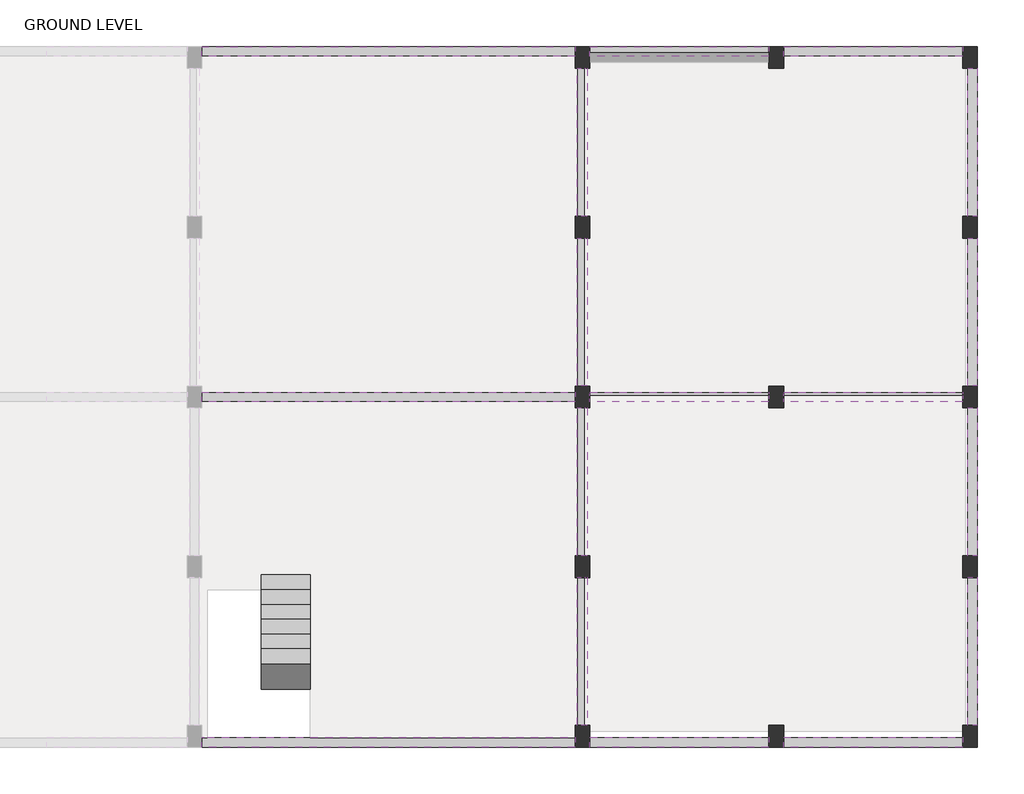
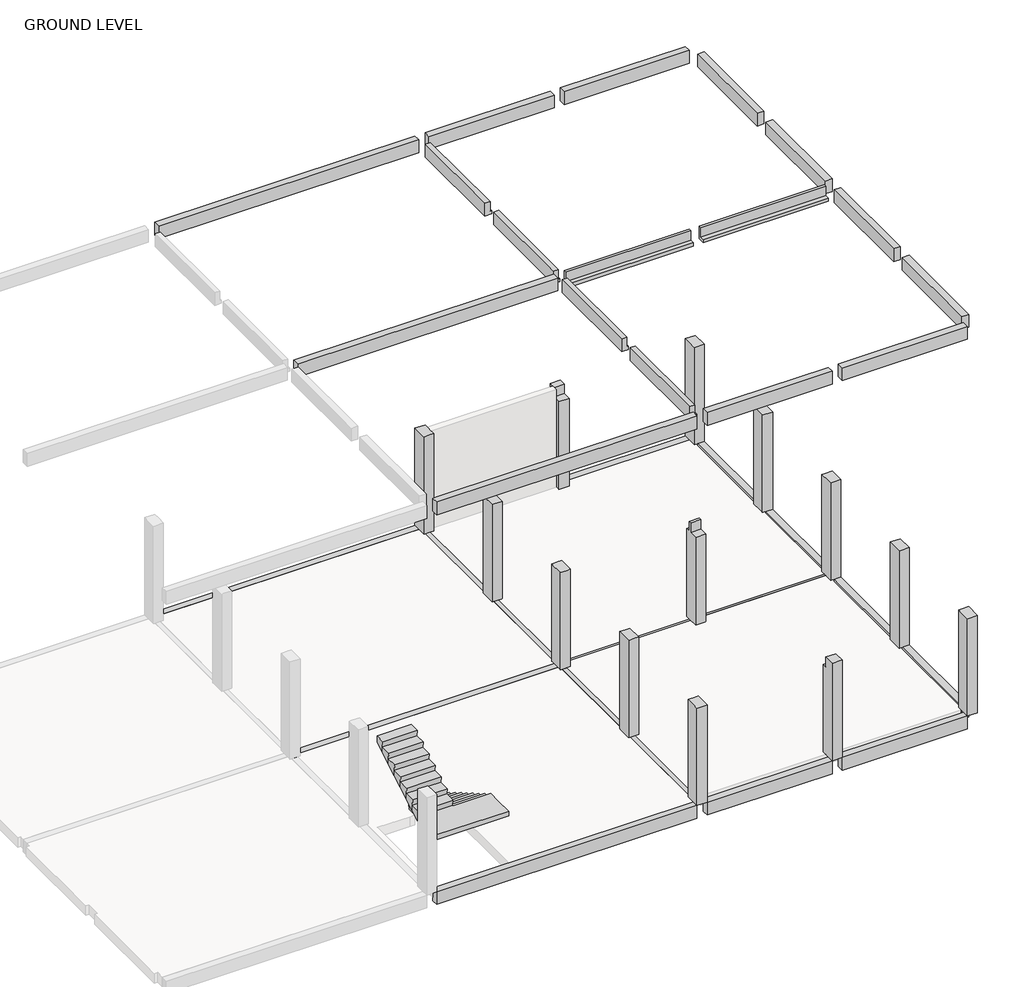
# One storey, part 2 of 2: 34 beams, 13 columns, 1 stair flight.
"""IFC4 building model written with IfcOpenShell, lengths in millimetres."""

from ifc_helpers import new_model, si_unit, frame, origin, place, context, project, spatial, polyline, outline, extrude, faceted_brep, element, save

model = new_model("IFC4")

# Units and contexts
model_context = context("Model", 3, world=origin())
ifc_project = project(units=[si_unit("LENGTHUNIT", "METRE", prefix="MILLI")], contexts=[model_context])

# Site, building, storey
site = spatial("IfcSite", under=ifc_project)
building = spatial("IfcBuilding", under=site)
storey = spatial("IfcBuildingStorey", under=building, Name="GROUND LEVEL", Elevation=0.0)

# Beams
placement = place(None, origin())
element("IfcBeam", 1, ObjectType="M_Concrete-Rectangular Beam : 200MMX400MM", at=placement, inside=storey, context=model_context, shape_type="Brep", body=[
    faceted_brep([(4019.3125983, 15797.7008557, 0.0), (4019.3125983, 15997.7008557, 0.0), (-3680.6874017, 15997.7008557, 0.0), (-3680.6874017, 15797.7008557, 0.0), (4019.3125983, 15797.7008557, -400.0), (4019.3125983, 15797.7008557, -300.0), (-3680.6874017, 15797.7008557, -300.0), (-3680.6874017, 15797.7008557, -400.0), (4019.3125983, 15997.7008557, -400.0), (-3680.6874017, 15997.7008557, -400.0)], [[[0, 1, 2, 3]], [[4, 5, 0, 3, 6, 7]], [[8, 4, 7, 9]], [[1, 8, 9, 2]], [[1, 0, 5, 4, 8]], [[2, 9, 7, 6, 3]]]),
])
element("IfcBeam", 2, ObjectType="M_Concrete-Rectangular Beam : 200MMX400MM", at=placement, inside=storey, context=model_context, shape_type="Brep", body=[
    faceted_brep([(8019.3125983, 15797.7008557, 0.0), (8019.3125983, 15997.7008557, 0.0), (4319.3125983, 15997.7008557, 0.0), (4319.3125983, 15797.7008557, 0.0), (8019.3125983, 15797.7008557, -400.0), (4319.3125983, 15797.7008557, -300.0), (4319.3125983, 15797.7008557, -400.0), (8019.3125983, 15997.7008557, -400.0), (4319.3125983, 15997.7008557, -400.0)], [[[0, 1, 2, 3]], [[4, 0, 3, 5, 6]], [[7, 4, 6, 8]], [[1, 7, 8, 2]], [[2, 8, 6, 5, 3]], [[1, 0, 4, 7]]]),
])
element("IfcBeam", 3, ObjectType="M_Concrete-Rectangular Beam : 200MMX400MM", at=placement, inside=storey, context=model_context, shape_type="Brep", body=[
    faceted_brep([(12019.3125983, 15797.7008557, 0.0), (12019.3125983, 15997.7008557, 0.0), (8319.3125983, 15997.7008557, 0.0), (8319.3125983, 15797.7008557, 0.0), (12019.3125983, 15797.7008557, -400.0), (12019.3125983, 15797.7008557, -300.0), (8319.3125983, 15797.7008557, -400.0), (12019.3125983, 15997.7008557, -400.0), (8319.3125983, 15997.7008557, -400.0)], [[[0, 1, 2, 3]], [[4, 5, 0, 3, 6]], [[7, 4, 6, 8]], [[1, 7, 8, 2]], [[2, 8, 6, 3]], [[1, 0, 5, 4, 7]]]),
])
element("IfcBeam", 4, ObjectType="M_Concrete-Rectangular Beam : 200MMX400MM", at=placement, inside=storey, context=model_context, shape_type="SweptSolid", body=[
    extrude(outline(polyline([(12319.3125983, 12497.7008557), (12119.3125983, 12497.7008557), (12119.3125983, 15547.7008557), (12319.3125983, 15547.7008557), (12319.3125983, 12497.7008557)])), frame((0.0, 0.0, -400.0), z_axis=(0.0, 0.0, 1.0), x_axis=(1.0, 0.0, 0.0)), (0.0, 0.0, 1.0), 400.0),
])
element("IfcBeam", 5, ObjectType="M_Concrete-Rectangular Beam : 200MMX400MM", at=placement, inside=storey, context=model_context, shape_type="SweptSolid", body=[
    extrude(outline(polyline([(12319.3125983, 1997.7008557), (12119.3125983, 1997.7008557), (12119.3125983, 5047.7008557), (12319.3125983, 5047.7008557), (12319.3125983, 1997.7008557)])), frame((0.0, 0.0, -400.0), z_axis=(0.0, 0.0, 1.0), x_axis=(1.0, 0.0, 0.0)), (0.0, 0.0, 1.0), 400.0),
])
element("IfcBeam", 6, ObjectType="M_Concrete-Rectangular Beam : 200MMX400MM", at=placement, inside=storey, context=model_context, shape_type="SweptSolid", body=[
    extrude(outline(polyline([(8319.3125983, 1547.7008557), (8319.3125983, 1747.7008557), (12019.3125983, 1747.7008557), (12019.3125983, 1547.7008557), (8319.3125983, 1547.7008557)])), frame((0.0, 0.0, -400.0), z_axis=(0.0, 0.0, 1.0), x_axis=(1.0, 0.0, 0.0)), (0.0, 0.0, 1.0), 400.0),
])
element("IfcBeam", 7, ObjectType="M_Concrete-Rectangular Beam : 200MMX400MM", at=placement, inside=storey, context=model_context, shape_type="SweptSolid", body=[
    extrude(outline(polyline([(8019.3125983, 1747.7008557), (8019.3125983, 1547.7008557), (4319.3125983, 1547.7008557), (4319.3125983, 1747.7008557), (8019.3125983, 1747.7008557)])), frame((0.0, 0.0, -400.0), z_axis=(0.0, 0.0, 1.0), x_axis=(1.0, 0.0, 0.0)), (0.0, 0.0, 1.0), 400.0),
])
element("IfcBeam", 8, ObjectType="M_Concrete-Rectangular Beam : 200MMX400MM", at=placement, inside=storey, context=model_context, shape_type="Brep", body=[
    faceted_brep([(-3680.6874017, 1747.7008557, 0.0), (-3680.6874017, 1547.7008557, 0.0), (4019.3125983, 1547.7008557, 0.0), (4019.3125983, 1747.7008557, 0.0), (-1437.0874017, 1747.7008557, 0.0), (-3570.6874017, 1747.7008557, 0.0), (-3680.6874017, 1747.7008557, -400.0), (-3680.6874017, 1747.7008557, -300.0), (4019.3125983, 1747.7008557, -300.0), (4019.3125983, 1747.7008557, -400.0), (-3680.6874017, 1547.7008557, -400.0), (4019.3125983, 1547.7008557, -400.0)], [[[0, 1, 2, 3, 4, 5]], [[6, 7, 0, 5, 4, 3, 8, 9]], [[10, 6, 9, 11]], [[1, 10, 11, 2]], [[1, 0, 7, 6, 10]], [[2, 11, 9, 8, 3]]]),
])
element("IfcBeam", 9, ObjectType="M_Concrete-Rectangular Beam : 200MMX400MM", at=placement, inside=storey, context=model_context, shape_type="Brep", body=[
    faceted_brep([(4019.3125983, 8872.7008557, 0.0), (-3680.6874017, 8872.7008557, 0.0), (-3680.6874017, 8672.7008557, 0.0), (4019.3125983, 8672.7008557, 0.0), (-3680.6874017, 8672.7008557, -300.0), (-3680.6874017, 8672.7008557, -400.0), (4019.3125983, 8672.7008557, -400.0), (4019.3125983, 8672.7008557, -300.0), (-3680.6874017, 8872.7008557, -400.0), (4019.3125983, 8872.7008557, -400.0), (4019.3125983, 8872.7008557, -300.0), (-3680.6874017, 8872.7008557, -300.0)], [[[0, 1, 2, 3]], [[3, 2, 4, 5, 6, 7]], [[6, 5, 8, 9]], [[1, 0, 10, 9, 8, 11]], [[8, 5, 4, 2, 1, 11]], [[0, 3, 7, 6, 9, 10]]]),
])
element("IfcBeam", 10, ObjectType="M_Concrete-Rectangular Beam : 200MMX400MM", at=placement, inside=storey, context=model_context, shape_type="Brep", body=[
    faceted_brep([(8019.3125983, 8872.7008557, 0.0), (4319.3125983, 8872.7008557, 0.0), (4319.3125983, 8797.7008557, 0.0), (8019.3125983, 8797.7008557, 0.0), (4319.3125983, 8672.7008557, -400.0), (8019.3125983, 8672.7008557, -400.0), (8019.3125983, 8672.7008557, -300.0), (4319.3125983, 8672.7008557, -300.0), (4319.3125983, 8872.7008557, -400.0), (8019.3125983, 8872.7008557, -400.0), (8019.3125983, 8872.7008557, -300.0), (4319.3125983, 8872.7008557, -300.0), (4319.3125983, 8797.7008557, -300.0), (8019.3125983, 8797.7008557, -300.0)], [[[0, 1, 2, 3]], [[4, 5, 6, 7]], [[5, 4, 8, 9]], [[1, 0, 10, 9, 8, 11]], [[8, 4, 7, 12, 2, 1, 11]], [[5, 9, 10, 0, 3, 13, 6]], [[13, 12, 7, 6]], [[12, 13, 3, 2]]]),
])
element("IfcBeam", 11, ObjectType="M_Concrete-Rectangular Beam : 200MMX400MM", at=placement, inside=storey, context=model_context, shape_type="Brep", body=[
    faceted_brep([(12019.3125983, 8872.7008557, 0.0), (8319.3125983, 8872.7008557, 0.0), (8319.3125983, 8797.7008557, 0.0), (12019.3125983, 8797.7008557, 0.0), (8319.3125983, 8672.7008557, -400.0), (12019.3125983, 8672.7008557, -400.0), (12019.3125983, 8672.7008557, -300.0), (8319.3125983, 8672.7008557, -300.0), (8319.3125983, 8872.7008557, -400.0), (12019.3125983, 8872.7008557, -400.0), (12019.3125983, 8872.7008557, -300.0), (8319.3125983, 8872.7008557, -300.0), (12019.3125983, 8797.7008557, -300.0), (8319.3125983, 8797.7008557, -300.0)], [[[0, 1, 2, 3]], [[4, 5, 6, 7]], [[5, 4, 8, 9]], [[1, 0, 10, 9, 8, 11]], [[5, 9, 10, 0, 3, 12, 6]], [[8, 4, 7, 13, 2, 1, 11]], [[12, 13, 7, 6]], [[13, 12, 3, 2]]]),
])
element("IfcBeam", 12, ObjectType="M_Concrete-Rectangular Beam : 200MMX400MM", at=placement, inside=storey, context=model_context, shape_type="SweptSolid", body=[
    extrude(outline(polyline([(12319.3125983, 5497.7008557), (12119.3125983, 5497.7008557), (12119.3125983, 8547.7008557), (12319.3125983, 8547.7008557), (12319.3125983, 5497.7008557)])), frame((0.0, 0.0, -400.0), z_axis=(0.0, 0.0, 1.0), x_axis=(1.0, 0.0, 0.0)), (0.0, 0.0, 1.0), 400.0),
])
element("IfcBeam", 13, ObjectType="M_Concrete-Rectangular Beam : 200MMX400MM", at=placement, inside=storey, context=model_context, shape_type="SweptSolid", body=[
    extrude(outline(polyline([(12119.3125983, 12047.7008557), (12319.3125983, 12047.7008557), (12319.3125983, 8997.7008557), (12119.3125983, 8997.7008557), (12119.3125983, 12047.7008557)])), frame((0.0, 0.0, -400.0), z_axis=(0.0, 0.0, 1.0), x_axis=(1.0, 0.0, 0.0)), (0.0, 0.0, 1.0), 400.0),
])
element("IfcBeam", 14, ObjectType="M_Concrete-Rectangular Beam : 200MMX400MM", at=placement, inside=storey, context=model_context, shape_type="Brep", body=[
    faceted_brep([(4069.3125983, 5047.7008557, 0.0), (4069.3125983, 1997.7008557, 0.0), (4219.3125983, 1997.7008557, 0.0), (4219.3125983, 5047.7008557, 0.0), (4269.3125983, 1997.7008557, -400.0), (4269.3125983, 5047.7008557, -400.0), (4269.3125983, 5047.7008557, -300.0), (4269.3125983, 1997.7008557, -300.0), (4069.3125983, 1997.7008557, -400.0), (4069.3125983, 5047.7008557, -400.0), (4069.3125983, 5047.7008557, -300.0), (4069.3125983, 1997.7008557, -300.0), (4219.3125983, 1997.7008557, -300.0), (4219.3125983, 5047.7008557, -300.0)], [[[0, 1, 2, 3]], [[4, 5, 6, 7]], [[5, 4, 8, 9]], [[1, 0, 10, 9, 8, 11]], [[8, 4, 7, 12, 2, 1, 11]], [[5, 9, 10, 0, 3, 13, 6]], [[13, 12, 7, 6]], [[12, 13, 3, 2]]]),
])
element("IfcBeam", 15, ObjectType="M_Concrete-Rectangular Beam : 200MMX400MM", at=placement, inside=storey, context=model_context, shape_type="Brep", body=[
    faceted_brep([(4069.3125983, 8547.7008557, 0.0), (4069.3125983, 5497.7008557, 0.0), (4219.3125983, 5497.7008557, 0.0), (4219.3125983, 8547.7008557, 0.0), (4269.3125983, 5497.7008557, -400.0), (4269.3125983, 8547.7008557, -400.0), (4269.3125983, 8547.7008557, -300.0), (4269.3125983, 5497.7008557, -300.0), (4069.3125983, 5497.7008557, -400.0), (4069.3125983, 8547.7008557, -400.0), (4069.3125983, 8547.7008557, -300.0), (4069.3125983, 5497.7008557, -300.0), (4219.3125983, 8547.7008557, -300.0), (4219.3125983, 5497.7008557, -300.0)], [[[0, 1, 2, 3]], [[4, 5, 6, 7]], [[5, 4, 8, 9]], [[1, 0, 10, 9, 8, 11]], [[5, 9, 10, 0, 3, 12, 6]], [[8, 4, 7, 13, 2, 1, 11]], [[12, 13, 7, 6]], [[13, 12, 3, 2]]]),
])
element("IfcBeam", 16, ObjectType="M_Concrete-Rectangular Beam : 200MMX400MM", at=placement, inside=storey, context=model_context, shape_type="Brep", body=[
    faceted_brep([(4069.3125983, 12047.7008557, 0.0), (4069.3125983, 8997.7008557, 0.0), (4219.3125983, 8997.7008557, 0.0), (4219.3125983, 12047.7008557, 0.0), (4269.3125983, 8997.7008557, -400.0), (4269.3125983, 12047.7008557, -400.0), (4269.3125983, 12047.7008557, -300.0), (4269.3125983, 8997.7008557, -300.0), (4069.3125983, 8997.7008557, -400.0), (4069.3125983, 12047.7008557, -400.0), (4069.3125983, 12047.7008557, -300.0), (4069.3125983, 8997.7008557, -300.0), (4219.3125983, 8997.7008557, -300.0), (4219.3125983, 12047.7008557, -300.0)], [[[0, 1, 2, 3]], [[4, 5, 6, 7]], [[5, 4, 8, 9]], [[1, 0, 10, 9, 8, 11]], [[8, 4, 7, 12, 2, 1, 11]], [[5, 9, 10, 0, 3, 13, 6]], [[13, 12, 7, 6]], [[12, 13, 3, 2]]]),
])
element("IfcBeam", 17, ObjectType="M_Concrete-Rectangular Beam : 200MMX400MM", at=placement, inside=storey, context=model_context, shape_type="Brep", body=[
    faceted_brep([(4069.3125983, 15547.7008557, 0.0), (4069.3125983, 12497.7008557, 0.0), (4219.3125983, 12497.7008557, 0.0), (4219.3125983, 15547.7008557, 0.0), (4269.3125983, 12497.7008557, -400.0), (4269.3125983, 15547.7008557, -400.0), (4269.3125983, 15547.7008557, -300.0), (4269.3125983, 12497.7008557, -300.0), (4069.3125983, 12497.7008557, -400.0), (4069.3125983, 15547.7008557, -400.0), (4069.3125983, 15547.7008557, -300.0), (4069.3125983, 12497.7008557, -300.0), (4219.3125983, 15547.7008557, -300.0), (4219.3125983, 12497.7008557, -300.0)], [[[0, 1, 2, 3]], [[4, 5, 6, 7]], [[5, 4, 8, 9]], [[1, 0, 10, 9, 8, 11]], [[5, 9, 10, 0, 3, 12, 6]], [[8, 4, 7, 13, 2, 1, 11]], [[12, 13, 7, 6]], [[13, 12, 3, 2]]]),
])
element("IfcBeam", 18, ObjectType="M_Concrete-Rectangular Beam : 200MMX400MM", at=placement, inside=storey, context=model_context, shape_type="Brep", body=[
    faceted_brep([(4019.3125983, 15797.7008557, 12192.0), (4019.3125983, 15997.7008557, 12192.0), (-3680.6874017, 15997.7008557, 12192.0), (-3680.6874017, 15797.7008557, 12192.0), (4019.3125983, 15797.7008557, 11792.0), (4019.3125983, 15797.7008557, 11892.0), (-3680.6874017, 15797.7008557, 11892.0), (-3680.6874017, 15797.7008557, 11792.0), (4019.3125983, 15997.7008557, 11792.0), (-3680.6874017, 15997.7008557, 11792.0)], [[[0, 1, 2, 3]], [[4, 5, 0, 3, 6, 7]], [[8, 4, 7, 9]], [[1, 8, 9, 2]], [[1, 0, 5, 4, 8]], [[2, 9, 7, 6, 3]]]),
])
element("IfcBeam", 19, ObjectType="M_Concrete-Rectangular Beam : 200MMX400MM", at=placement, inside=storey, context=model_context, shape_type="Brep", body=[
    faceted_brep([(8019.3125983, 15797.7008557, 12192.0), (8019.3125983, 15997.7008557, 12192.0), (4319.3125983, 15997.7008557, 12192.0), (4319.3125983, 15797.7008557, 12192.0), (8019.3125983, 15797.7008557, 11792.0), (4319.3125983, 15797.7008557, 11892.0), (4319.3125983, 15797.7008557, 11792.0), (8019.3125983, 15997.7008557, 11792.0), (4319.3125983, 15997.7008557, 11792.0)], [[[0, 1, 2, 3]], [[4, 0, 3, 5, 6]], [[7, 4, 6, 8]], [[1, 7, 8, 2]], [[2, 8, 6, 5, 3]], [[1, 0, 4, 7]]]),
])
element("IfcBeam", 20, ObjectType="M_Concrete-Rectangular Beam : 200MMX400MM", at=placement, inside=storey, context=model_context, shape_type="Brep", body=[
    faceted_brep([(12019.3125983, 15797.7008557, 12192.0), (12019.3125983, 15997.7008557, 12192.0), (8319.3125983, 15997.7008557, 12192.0), (8319.3125983, 15797.7008557, 12192.0), (12019.3125983, 15797.7008557, 11792.0), (12019.3125983, 15797.7008557, 11892.0), (8319.3125983, 15797.7008557, 11792.0), (12019.3125983, 15997.7008557, 11792.0), (8319.3125983, 15997.7008557, 11792.0)], [[[0, 1, 2, 3]], [[4, 5, 0, 3, 6]], [[7, 4, 6, 8]], [[1, 7, 8, 2]], [[2, 8, 6, 3]], [[1, 0, 5, 4, 7]]]),
])
element("IfcBeam", 21, ObjectType="M_Concrete-Rectangular Beam : 200MMX400MM", at=placement, inside=storey, context=model_context, shape_type="SweptSolid", body=[
    extrude(outline(polyline([(12319.3125983, 12497.7008557), (12119.3125983, 12497.7008557), (12119.3125983, 15547.7008557), (12319.3125983, 15547.7008557), (12319.3125983, 12497.7008557)])), frame((0.0, 0.0, 11792.0), z_axis=(0.0, 0.0, 1.0), x_axis=(1.0, 0.0, 0.0)), (0.0, 0.0, 1.0), 400.0),
])
element("IfcBeam", 22, ObjectType="M_Concrete-Rectangular Beam : 200MMX400MM", at=placement, inside=storey, context=model_context, shape_type="SweptSolid", body=[
    extrude(outline(polyline([(12319.3125983, 1997.7008557), (12119.3125983, 1997.7008557), (12119.3125983, 5047.7008557), (12319.3125983, 5047.7008557), (12319.3125983, 1997.7008557)])), frame((0.0, 0.0, 11792.0), z_axis=(0.0, 0.0, 1.0), x_axis=(1.0, 0.0, 0.0)), (0.0, 0.0, 1.0), 400.0),
])
element("IfcBeam", 23, ObjectType="M_Concrete-Rectangular Beam : 200MMX400MM", at=placement, inside=storey, context=model_context, shape_type="SweptSolid", body=[
    extrude(outline(polyline([(8319.3125983, 1547.7008557), (8319.3125983, 1747.7008557), (12019.3125983, 1747.7008557), (12019.3125983, 1547.7008557), (8319.3125983, 1547.7008557)])), frame((0.0, 0.0, 11792.0), z_axis=(0.0, 0.0, 1.0), x_axis=(1.0, 0.0, 0.0)), (0.0, 0.0, 1.0), 400.0),
])
element("IfcBeam", 24, ObjectType="M_Concrete-Rectangular Beam : 200MMX400MM", at=placement, inside=storey, context=model_context, shape_type="SweptSolid", body=[
    extrude(outline(polyline([(8019.3125983, 1747.7008557), (8019.3125983, 1547.7008557), (4319.3125983, 1547.7008557), (4319.3125983, 1747.7008557), (8019.3125983, 1747.7008557)])), frame((0.0, 0.0, 11792.0), z_axis=(0.0, 0.0, 1.0), x_axis=(1.0, 0.0, 0.0)), (0.0, 0.0, 1.0), 400.0),
])
element("IfcBeam", 25, ObjectType="M_Concrete-Rectangular Beam : 200MMX400MM", at=placement, inside=storey, context=model_context, shape_type="Brep", body=[
    faceted_brep([(-3680.6874017, 1747.7008557, 12192.0), (-3680.6874017, 1547.7008557, 12192.0), (4019.3125983, 1547.7008557, 12192.0), (4019.3125983, 1747.7008557, 12192.0), (-1437.0874017, 1747.7008557, 12192.0), (-3570.6874017, 1747.7008557, 12192.0), (-3680.6874017, 1747.7008557, 11792.0), (-3680.6874017, 1747.7008557, 11892.0), (4019.3125983, 1747.7008557, 11892.0), (4019.3125983, 1747.7008557, 11792.0), (-3680.6874017, 1547.7008557, 11792.0), (4019.3125983, 1547.7008557, 11792.0)], [[[0, 1, 2, 3, 4, 5]], [[6, 7, 0, 5, 4, 3, 8, 9]], [[10, 6, 9, 11]], [[1, 10, 11, 2]], [[1, 0, 7, 6, 10]], [[2, 11, 9, 8, 3]]]),
])
element("IfcBeam", 26, ObjectType="M_Concrete-Rectangular Beam : 200MMX400MM", at=placement, inside=storey, context=model_context, shape_type="Brep", body=[
    faceted_brep([(4019.3125983, 8872.7008557, 12192.0), (-3680.6874017, 8872.7008557, 12192.0), (-3680.6874017, 8672.7008557, 12192.0), (4019.3125983, 8672.7008557, 12192.0), (-3680.6874017, 8672.7008557, 11892.0), (-3680.6874017, 8672.7008557, 11792.0), (4019.3125983, 8672.7008557, 11792.0), (4019.3125983, 8672.7008557, 11892.0), (-3680.6874017, 8872.7008557, 11792.0), (4019.3125983, 8872.7008557, 11792.0), (4019.3125983, 8872.7008557, 11892.0), (-3680.6874017, 8872.7008557, 11892.0)], [[[0, 1, 2, 3]], [[3, 2, 4, 5, 6, 7]], [[6, 5, 8, 9]], [[1, 0, 10, 9, 8, 11]], [[8, 5, 4, 2, 1, 11]], [[0, 3, 7, 6, 9, 10]]]),
])
element("IfcBeam", 27, ObjectType="M_Concrete-Rectangular Beam : 200MMX400MM", at=placement, inside=storey, context=model_context, shape_type="Brep", body=[
    faceted_brep([(8019.3125983, 8872.7008557, 12192.0), (4319.3125983, 8872.7008557, 12192.0), (4319.3125983, 8797.7008557, 12192.0), (8019.3125983, 8797.7008557, 12192.0), (4319.3125983, 8672.7008557, 11792.0), (8019.3125983, 8672.7008557, 11792.0), (8019.3125983, 8672.7008557, 11892.0), (4319.3125983, 8672.7008557, 11892.0), (4319.3125983, 8872.7008557, 11792.0), (8019.3125983, 8872.7008557, 11792.0), (8019.3125983, 8872.7008557, 11892.0), (4319.3125983, 8872.7008557, 11892.0), (4319.3125983, 8797.7008557, 11892.0), (8019.3125983, 8797.7008557, 11892.0)], [[[0, 1, 2, 3]], [[4, 5, 6, 7]], [[5, 4, 8, 9]], [[1, 0, 10, 9, 8, 11]], [[8, 4, 7, 12, 2, 1, 11]], [[5, 9, 10, 0, 3, 13, 6]], [[13, 12, 7, 6]], [[12, 13, 3, 2]]]),
])
element("IfcBeam", 28, ObjectType="M_Concrete-Rectangular Beam : 200MMX400MM", at=placement, inside=storey, context=model_context, shape_type="Brep", body=[
    faceted_brep([(12019.3125983, 8872.7008557, 12192.0), (8319.3125983, 8872.7008557, 12192.0), (8319.3125983, 8797.7008557, 12192.0), (12019.3125983, 8797.7008557, 12192.0), (8319.3125983, 8672.7008557, 11792.0), (12019.3125983, 8672.7008557, 11792.0), (12019.3125983, 8672.7008557, 11892.0), (8319.3125983, 8672.7008557, 11892.0), (8319.3125983, 8872.7008557, 11792.0), (12019.3125983, 8872.7008557, 11792.0), (12019.3125983, 8872.7008557, 11892.0), (8319.3125983, 8872.7008557, 11892.0), (12019.3125983, 8797.7008557, 11892.0), (8319.3125983, 8797.7008557, 11892.0)], [[[0, 1, 2, 3]], [[4, 5, 6, 7]], [[5, 4, 8, 9]], [[1, 0, 10, 9, 8, 11]], [[5, 9, 10, 0, 3, 12, 6]], [[8, 4, 7, 13, 2, 1, 11]], [[12, 13, 7, 6]], [[13, 12, 3, 2]]]),
])
element("IfcBeam", 29, ObjectType="M_Concrete-Rectangular Beam : 200MMX400MM", at=placement, inside=storey, context=model_context, shape_type="SweptSolid", body=[
    extrude(outline(polyline([(12319.3125983, 5497.7008557), (12119.3125983, 5497.7008557), (12119.3125983, 8547.7008557), (12319.3125983, 8547.7008557), (12319.3125983, 5497.7008557)])), frame((0.0, 0.0, 11792.0), z_axis=(0.0, 0.0, 1.0), x_axis=(1.0, 0.0, 0.0)), (0.0, 0.0, 1.0), 400.0),
])
element("IfcBeam", 30, ObjectType="M_Concrete-Rectangular Beam : 200MMX400MM", at=placement, inside=storey, context=model_context, shape_type="SweptSolid", body=[
    extrude(outline(polyline([(12119.3125983, 12047.7008557), (12319.3125983, 12047.7008557), (12319.3125983, 8997.7008557), (12119.3125983, 8997.7008557), (12119.3125983, 12047.7008557)])), frame((0.0, 0.0, 11792.0), z_axis=(0.0, 0.0, 1.0), x_axis=(1.0, 0.0, 0.0)), (0.0, 0.0, 1.0), 400.0),
])
element("IfcBeam", 31, ObjectType="M_Concrete-Rectangular Beam : 200MMX400MM", at=placement, inside=storey, context=model_context, shape_type="Brep", body=[
    faceted_brep([(4069.3125983, 5047.7008557, 12192.0), (4069.3125983, 1997.7008557, 12192.0), (4219.3125983, 1997.7008557, 12192.0), (4219.3125983, 5047.7008557, 12192.0), (4269.3125983, 1997.7008557, 11792.0), (4269.3125983, 5047.7008557, 11792.0), (4269.3125983, 5047.7008557, 11892.0), (4269.3125983, 1997.7008557, 11892.0), (4069.3125983, 1997.7008557, 11792.0), (4069.3125983, 5047.7008557, 11792.0), (4069.3125983, 5047.7008557, 11892.0), (4069.3125983, 1997.7008557, 11892.0), (4219.3125983, 1997.7008557, 11892.0), (4219.3125983, 5047.7008557, 11892.0)], [[[0, 1, 2, 3]], [[4, 5, 6, 7]], [[5, 4, 8, 9]], [[1, 0, 10, 9, 8, 11]], [[8, 4, 7, 12, 2, 1, 11]], [[5, 9, 10, 0, 3, 13, 6]], [[13, 12, 7, 6]], [[12, 13, 3, 2]]]),
])
element("IfcBeam", 32, ObjectType="M_Concrete-Rectangular Beam : 200MMX400MM", at=placement, inside=storey, context=model_context, shape_type="Brep", body=[
    faceted_brep([(4069.3125983, 8547.7008557, 12192.0), (4069.3125983, 5497.7008557, 12192.0), (4219.3125983, 5497.7008557, 12192.0), (4219.3125983, 8547.7008557, 12192.0), (4269.3125983, 5497.7008557, 11792.0), (4269.3125983, 8547.7008557, 11792.0), (4269.3125983, 8547.7008557, 11892.0), (4269.3125983, 5497.7008557, 11892.0), (4069.3125983, 5497.7008557, 11792.0), (4069.3125983, 8547.7008557, 11792.0), (4069.3125983, 8547.7008557, 11892.0), (4069.3125983, 5497.7008557, 11892.0), (4219.3125983, 8547.7008557, 11892.0), (4219.3125983, 5497.7008557, 11892.0)], [[[0, 1, 2, 3]], [[4, 5, 6, 7]], [[5, 4, 8, 9]], [[1, 0, 10, 9, 8, 11]], [[5, 9, 10, 0, 3, 12, 6]], [[8, 4, 7, 13, 2, 1, 11]], [[12, 13, 7, 6]], [[13, 12, 3, 2]]]),
])
element("IfcBeam", 33, ObjectType="M_Concrete-Rectangular Beam : 200MMX400MM", at=placement, inside=storey, context=model_context, shape_type="Brep", body=[
    faceted_brep([(4069.3125983, 12047.7008557, 12192.0), (4069.3125983, 8997.7008557, 12192.0), (4219.3125983, 8997.7008557, 12192.0), (4219.3125983, 12047.7008557, 12192.0), (4269.3125983, 8997.7008557, 11792.0), (4269.3125983, 12047.7008557, 11792.0), (4269.3125983, 12047.7008557, 11892.0), (4269.3125983, 8997.7008557, 11892.0), (4069.3125983, 8997.7008557, 11792.0), (4069.3125983, 12047.7008557, 11792.0), (4069.3125983, 12047.7008557, 11892.0), (4069.3125983, 8997.7008557, 11892.0), (4219.3125983, 8997.7008557, 11892.0), (4219.3125983, 12047.7008557, 11892.0)], [[[0, 1, 2, 3]], [[4, 5, 6, 7]], [[5, 4, 8, 9]], [[1, 0, 10, 9, 8, 11]], [[8, 4, 7, 12, 2, 1, 11]], [[5, 9, 10, 0, 3, 13, 6]], [[13, 12, 7, 6]], [[12, 13, 3, 2]]]),
])
element("IfcBeam", 34, ObjectType="M_Concrete-Rectangular Beam : 200MMX400MM", at=placement, inside=storey, context=model_context, shape_type="Brep", body=[
    faceted_brep([(4069.3125983, 15547.7008557, 12192.0), (4069.3125983, 12497.7008557, 12192.0), (4219.3125983, 12497.7008557, 12192.0), (4219.3125983, 15547.7008557, 12192.0), (4269.3125983, 12497.7008557, 11792.0), (4269.3125983, 15547.7008557, 11792.0), (4269.3125983, 15547.7008557, 11892.0), (4269.3125983, 12497.7008557, 11892.0), (4069.3125983, 12497.7008557, 11792.0), (4069.3125983, 15547.7008557, 11792.0), (4069.3125983, 15547.7008557, 11892.0), (4069.3125983, 12497.7008557, 11892.0), (4219.3125983, 15547.7008557, 11892.0), (4219.3125983, 12497.7008557, 11892.0)], [[[0, 1, 2, 3]], [[4, 5, 6, 7]], [[5, 4, 8, 9]], [[1, 0, 10, 9, 8, 11]], [[5, 9, 10, 0, 3, 12, 6]], [[8, 4, 7, 13, 2, 1, 11]], [[12, 13, 7, 6]], [[13, 12, 3, 2]]]),
])

# Columns
element("IfcColumn", 35, ObjectType="M_Concrete-Rectangular-Column : 300 x 450mm", at=placement, inside=storey, context=model_context, shape_type="Brep", body=[
    faceted_brep([(4319.3125983, 15997.7008557, 0.0), (4319.3125983, 15547.7008557, 0.0), (4019.3125983, 15547.7008557, 0.0), (4019.3125983, 15997.7008557, 0.0), (4319.3125983, 15997.7008557, 3048.0), (4319.3125983, 15797.7008557, 3048.0), (4319.3125983, 15547.7008557, 3048.0), (4319.3125983, 15547.7008557, 2748.0), (4219.3125983, 15547.7008557, 3048.0), (4069.3125983, 15547.7008557, 3048.0), (4019.3125983, 15547.7008557, 3048.0), (4019.3125983, 15547.7008557, 2748.0), (4019.3125983, 15797.7008557, 3048.0), (4019.3125983, 15997.7008557, 3048.0)], [[[0, 1, 2, 3]], [[1, 0, 4, 5, 6, 7]], [[2, 1, 7, 6, 8, 9, 10, 11]], [[3, 2, 11, 10, 12, 13]], [[0, 3, 13, 4]], [[4, 13, 12, 10, 9, 8, 6, 5]]]),
])
element("IfcColumn", 36, ObjectType="M_Concrete-Rectangular-Column : 300 x 450mm", at=placement, inside=storey, context=model_context, shape_type="Brep", body=[
    faceted_brep([(4319.3125983, 8997.7008557, 0.0), (4319.3125983, 8547.7008557, 0.0), (4019.3125983, 8547.7008557, 0.0), (4019.3125983, 8997.7008557, 0.0), (4319.3125983, 8997.7008557, 2748.0), (4319.3125983, 8997.7008557, 3048.0), (4319.3125983, 8872.7008557, 3048.0), (4319.3125983, 8797.7008557, 3048.0), (4319.3125983, 8547.7008557, 3048.0), (4319.3125983, 8547.7008557, 2748.0), (4219.3125983, 8547.7008557, 3048.0), (4069.3125983, 8547.7008557, 3048.0), (4019.3125983, 8547.7008557, 3048.0), (4019.3125983, 8547.7008557, 2748.0), (4019.3125983, 8672.7008557, 3048.0), (4019.3125983, 8872.7008557, 3048.0), (4019.3125983, 8997.7008557, 3048.0), (4019.3125983, 8997.7008557, 2748.0), (4069.3125983, 8997.7008557, 3048.0), (4219.3125983, 8997.7008557, 3048.0)], [[[0, 1, 2, 3]], [[1, 0, 4, 5, 6, 7, 8, 9]], [[2, 1, 9, 8, 10, 11, 12, 13]], [[3, 2, 13, 12, 14, 15, 16, 17]], [[0, 3, 17, 16, 18, 19, 5, 4]], [[18, 16, 15, 14, 12, 11, 10, 8, 7, 6, 5, 19]]]),
])
element("IfcColumn", 37, ObjectType="M_Concrete-Rectangular-Column : 300 x 450mm", at=placement, inside=storey, context=model_context, shape_type="Brep", body=[
    faceted_brep([(4319.3125983, 1997.7008557, 0.0), (4319.3125983, 1547.7008557, 0.0), (4019.3125983, 1547.7008557, 0.0), (4019.3125983, 1997.7008557, 0.0), (4319.3125983, 1997.7008557, 2748.0), (4319.3125983, 1997.7008557, 3048.0), (4319.3125983, 1872.7008557, 3048.0), (4319.3125983, 1547.7008557, 3048.0), (4019.3125983, 1547.7008557, 3048.0), (4019.3125983, 1747.7008557, 3048.0), (4019.3125983, 1997.7008557, 3048.0), (4019.3125983, 1997.7008557, 2748.0), (4069.3125983, 1997.7008557, 3048.0), (4219.3125983, 1997.7008557, 3048.0)], [[[0, 1, 2, 3]], [[1, 0, 4, 5, 6, 7]], [[2, 1, 7, 8]], [[3, 2, 8, 9, 10, 11]], [[0, 3, 11, 10, 12, 13, 5, 4]], [[8, 7, 6, 5, 13, 12, 10, 9]]]),
])
element("IfcColumn", 38, ObjectType="M_Concrete-Rectangular-Column : 300 x 450mm", at=placement, inside=storey, context=model_context, shape_type="SweptSolid", body=[
    extrude(outline(polyline([(15997.7008557, 0.0), (15547.7008557, 0.0), (15547.7008557, 2748.0), (15797.7008557, 2748.0), (15797.7008557, 3048.0), (15997.7008557, 3048.0), (15997.7008557, 0.0)])), frame((8019.3125983, 0.0, 0.0), z_axis=(1.0, 0.0, 0.0), x_axis=(0.0, 1.0, 0.0)), (0.0, 0.0, 1.0), 300.0),
])
element("IfcColumn", 39, ObjectType="M_Concrete-Rectangular-Column : 300 x 450mm", at=placement, inside=storey, context=model_context, shape_type="SweptSolid", body=[
    extrude(outline(polyline([(1997.7008557, 0.0), (1547.7008557, 0.0), (1547.7008557, 3048.0), (1872.7008557, 3048.0), (1872.7008557, 2748.0), (1997.7008557, 2748.0), (1997.7008557, 0.0)])), frame((8019.3125983, 0.0, 0.0), z_axis=(1.0, 0.0, 0.0), x_axis=(0.0, 1.0, 0.0)), (0.0, 0.0, 1.0), 300.0),
])
element("IfcColumn", 40, ObjectType="M_Concrete-Rectangular-Column : 300 x 450mm", at=placement, inside=storey, context=model_context, shape_type="Brep", body=[
    faceted_brep([(12319.3125983, 12497.7008557, 0.0), (12319.3125983, 12047.7008557, 0.0), (12019.3125983, 12047.7008557, 0.0), (12019.3125983, 12497.7008557, 0.0), (12319.3125983, 12497.7008557, 3048.0), (12319.3125983, 12047.7008557, 3048.0), (12069.3125983, 12047.7008557, 3048.0), (12019.3125983, 12047.7008557, 3048.0), (12019.3125983, 12047.7008557, 2748.0), (12019.3125983, 12497.7008557, 3048.0), (12019.3125983, 12497.7008557, 2748.0), (12069.3125983, 12497.7008557, 3048.0)], [[[0, 1, 2, 3]], [[1, 0, 4, 5]], [[2, 1, 5, 6, 7, 8]], [[3, 2, 8, 7, 9, 10]], [[0, 3, 10, 9, 11, 4]], [[5, 4, 11, 9, 7, 6]]]),
])
element("IfcColumn", 41, ObjectType="M_Concrete-Rectangular-Column : 300 x 450mm", at=placement, inside=storey, context=model_context, shape_type="Brep", body=[
    faceted_brep([(12319.3125983, 5497.7008557, 0.0), (12319.3125983, 5047.7008557, 0.0), (12019.3125983, 5047.7008557, 0.0), (12019.3125983, 5497.7008557, 0.0), (12319.3125983, 5497.7008557, 3048.0), (12319.3125983, 5047.7008557, 3048.0), (12069.3125983, 5047.7008557, 3048.0), (12019.3125983, 5047.7008557, 3048.0), (12019.3125983, 5047.7008557, 2748.0), (12019.3125983, 5497.7008557, 3048.0), (12019.3125983, 5497.7008557, 2748.0), (12069.3125983, 5497.7008557, 3048.0)], [[[0, 1, 2, 3]], [[1, 0, 4, 5]], [[2, 1, 5, 6, 7, 8]], [[3, 2, 8, 7, 9, 10]], [[0, 3, 10, 9, 11, 4]], [[5, 4, 11, 9, 7, 6]]]),
])
element("IfcColumn", 42, ObjectType="M_Concrete-Rectangular-Column : 300 x 450mm", at=placement, inside=storey, context=model_context, shape_type="Brep", body=[
    faceted_brep([(12319.3125983, 15997.7008557, 0.0), (12319.3125983, 15547.7008557, 0.0), (12019.3125983, 15547.7008557, 0.0), (12019.3125983, 15997.7008557, 0.0), (12319.3125983, 15997.7008557, 3048.0), (12319.3125983, 15547.7008557, 3048.0), (12069.3125983, 15547.7008557, 3048.0), (12019.3125983, 15547.7008557, 3048.0), (12019.3125983, 15547.7008557, 2748.0), (12019.3125983, 15797.7008557, 3048.0), (12019.3125983, 15997.7008557, 3048.0)], [[[0, 1, 2, 3]], [[1, 0, 4, 5]], [[2, 1, 5, 6, 7, 8]], [[3, 2, 8, 7, 9, 10]], [[0, 3, 10, 4]], [[5, 4, 10, 9, 7, 6]]]),
])
element("IfcColumn", 43, ObjectType="M_Concrete-Rectangular-Column : 300 x 450mm", at=placement, inside=storey, context=model_context, shape_type="Brep", body=[
    faceted_brep([(12319.3125983, 1997.7008557, 0.0), (12319.3125983, 1547.7008557, 0.0), (12019.3125983, 1547.7008557, 0.0), (12019.3125983, 1997.7008557, 0.0), (12319.3125983, 1997.7008557, 3048.0), (12319.3125983, 1547.7008557, 3048.0), (12019.3125983, 1547.7008557, 3048.0), (12019.3125983, 1872.7008557, 3048.0), (12019.3125983, 1997.7008557, 3048.0), (12019.3125983, 1997.7008557, 2748.0), (12069.3125983, 1997.7008557, 3048.0)], [[[0, 1, 2, 3]], [[1, 0, 4, 5]], [[2, 1, 5, 6]], [[3, 2, 6, 7, 8, 9]], [[0, 3, 9, 8, 10, 4]], [[5, 4, 10, 8, 7, 6]]]),
])
element("IfcColumn", 44, ObjectType="M_Concrete-Rectangular-Column : 300 x 450mm", at=placement, inside=storey, context=model_context, shape_type="Brep", body=[
    faceted_brep([(12319.3125983, 8997.7008557, 0.0), (12319.3125983, 8547.7008557, 0.0), (12019.3125983, 8547.7008557, 0.0), (12019.3125983, 8997.7008557, 0.0), (12319.3125983, 8997.7008557, 3048.0), (12319.3125983, 8547.7008557, 3048.0), (12069.3125983, 8547.7008557, 3048.0), (12019.3125983, 8547.7008557, 3048.0), (12019.3125983, 8547.7008557, 2748.0), (12019.3125983, 8797.7008557, 3048.0), (12019.3125983, 8872.7008557, 3048.0), (12019.3125983, 8997.7008557, 3048.0), (12019.3125983, 8997.7008557, 2748.0), (12069.3125983, 8997.7008557, 3048.0)], [[[0, 1, 2, 3]], [[1, 0, 4, 5]], [[2, 1, 5, 6, 7, 8]], [[3, 2, 8, 7, 9, 10, 11, 12]], [[0, 3, 12, 11, 13, 4]], [[5, 4, 13, 11, 10, 9, 7, 6]]]),
])
element("IfcColumn", 45, ObjectType="M_Concrete-Rectangular-Column : 300 x 450mm", at=placement, inside=storey, context=model_context, shape_type="Brep", body=[
    faceted_brep([(8319.3125983, 8997.7008557, 0.0), (8319.3125983, 8547.7008557, 0.0), (8019.3125983, 8547.7008557, 0.0), (8019.3125983, 8997.7008557, 0.0), (8319.3125983, 8997.7008557, 2748.0), (8319.3125983, 8872.7008557, 2748.0), (8319.3125983, 8872.7008557, 3048.0), (8319.3125983, 8797.7008557, 3048.0), (8319.3125983, 8797.7008557, 2748.0), (8319.3125983, 8547.7008557, 2748.0), (8019.3125983, 8547.7008557, 2748.0), (8019.3125983, 8672.7008557, 2748.0), (8019.3125983, 8797.7008557, 2748.0), (8019.3125983, 8797.7008557, 3048.0), (8019.3125983, 8872.7008557, 3048.0), (8019.3125983, 8872.7008557, 2748.0), (8019.3125983, 8997.7008557, 2748.0)], [[[0, 1, 2, 3]], [[1, 0, 4, 5, 6, 7, 8, 9]], [[2, 1, 9, 10]], [[3, 2, 10, 11, 12, 13, 14, 15, 16]], [[0, 3, 16, 4]], [[14, 13, 7, 6]], [[8, 12, 11, 10, 9]], [[5, 15, 14, 6]], [[12, 8, 7, 13]], [[15, 5, 4, 16]]]),
])
element("IfcColumn", 46, ObjectType="M_Concrete-Rectangular-Column : 300 x 450mm", at=placement, inside=storey, context=model_context, shape_type="Brep", body=[
    faceted_brep([(4319.3125983, 12497.7008557, 0.0), (4319.3125983, 12047.7008557, 0.0), (4019.3125983, 12047.7008557, 0.0), (4019.3125983, 12497.7008557, 0.0), (4319.3125983, 12497.7008557, 2748.0), (4319.3125983, 12497.7008557, 3048.0), (4319.3125983, 12047.7008557, 3048.0), (4319.3125983, 12047.7008557, 2748.0), (4219.3125983, 12047.7008557, 3048.0), (4069.3125983, 12047.7008557, 3048.0), (4019.3125983, 12047.7008557, 3048.0), (4019.3125983, 12047.7008557, 2748.0), (4019.3125983, 12497.7008557, 3048.0), (4019.3125983, 12497.7008557, 2748.0), (4069.3125983, 12497.7008557, 3048.0), (4219.3125983, 12497.7008557, 3048.0)], [[[0, 1, 2, 3]], [[1, 0, 4, 5, 6, 7]], [[2, 1, 7, 6, 8, 9, 10, 11]], [[3, 2, 11, 10, 12, 13]], [[0, 3, 13, 12, 14, 15, 5, 4]], [[6, 5, 15, 14, 12, 10, 9, 8]]]),
])
element("IfcColumn", 47, ObjectType="M_Concrete-Rectangular-Column : 300 x 450mm", at=placement, inside=storey, context=model_context, shape_type="Brep", body=[
    faceted_brep([(4319.3125983, 5497.7008557, 0.0), (4319.3125983, 5047.7008557, 0.0), (4019.3125983, 5047.7008557, 0.0), (4019.3125983, 5497.7008557, 0.0), (4319.3125983, 5497.7008557, 2748.0), (4319.3125983, 5497.7008557, 3048.0), (4319.3125983, 5047.7008557, 3048.0), (4319.3125983, 5047.7008557, 2748.0), (4219.3125983, 5047.7008557, 3048.0), (4069.3125983, 5047.7008557, 3048.0), (4019.3125983, 5047.7008557, 3048.0), (4019.3125983, 5047.7008557, 2748.0), (4019.3125983, 5497.7008557, 3048.0), (4019.3125983, 5497.7008557, 2748.0), (4069.3125983, 5497.7008557, 3048.0), (4219.3125983, 5497.7008557, 3048.0)], [[[0, 1, 2, 3]], [[1, 0, 4, 5, 6, 7]], [[2, 1, 7, 6, 8, 9, 10, 11]], [[3, 2, 11, 10, 12, 13]], [[0, 3, 13, 12, 14, 15, 5, 4]], [[6, 5, 15, 14, 12, 10, 9, 8]]]),
])

# Stair flight
element("IfcStairFlight", 48, ObjectType="25 mm Nosing", at=placement, inside=storey, context=model_context, shape_type="Brep", body=[
    faceted_brep([(-1437.0874017, 5100.5008557, 179.2941176), (-2453.0874017, 5100.5008557, 179.2941176), (-2453.0874017, 4770.7008557, 179.2941176), (-1437.0874017, 4770.7008557, 179.2941176), (-1437.0874017, 4770.7008557, 5.2669154), (-1437.0874017, 4779.6546118, 0.0), (-1437.0874017, 5075.5008557, 0.0), (-2453.0874017, 5075.5008557, 0.0), (-2453.0874017, 4779.6546118, 0.0), (-2453.0874017, 4770.7008557, 5.2669154), (-1437.0874017, 4795.7008557, 358.5882353), (-2453.0874017, 4795.7008557, 358.5882353), (-2453.0874017, 4465.9008557, 358.5882353), (-1437.0874017, 4465.9008557, 358.5882353), (-1437.0874017, 4465.9008557, 184.561033), (-2453.0874017, 4465.9008557, 184.561033), (-1437.0874017, 4490.9008557, 537.8823529), (-2453.0874017, 4490.9008557, 537.8823529), (-2453.0874017, 4161.1008557, 537.8823529), (-1437.0874017, 4161.1008557, 537.8823529), (-1437.0874017, 4161.1008557, 363.8551507), (-2453.0874017, 4161.1008557, 363.8551507), (-1437.0874017, 4186.1008557, 717.1764706), (-2453.0874017, 4186.1008557, 717.1764706), (-2453.0874017, 3856.3008557, 717.1764706), (-1437.0874017, 3856.3008557, 717.1764706), (-1437.0874017, 3856.3008557, 543.1492683), (-2453.0874017, 3856.3008557, 543.1492683), (-1437.0874017, 3881.3008557, 896.4705882), (-2453.0874017, 3881.3008557, 896.4705882), (-2453.0874017, 3551.5008557, 896.4705882), (-1437.0874017, 3551.5008557, 896.4705882), (-1437.0874017, 3551.5008557, 722.443386), (-2453.0874017, 3551.5008557, 722.443386), (-1437.0874017, 3576.5008557, 1075.7647059), (-2453.0874017, 3576.5008557, 1075.7647059), (-2453.0874017, 3246.7008557, 1075.7647059), (-1437.0874017, 3246.7008557, 1075.7647059), (-1437.0874017, 3246.7008557, 901.7375036), (-2453.0874017, 3246.7008557, 901.7375036), (-1437.0874017, 3271.7008557, 1255.0588235), (-2453.0874017, 3271.7008557, 1255.0588235), (-2453.0874017, 2941.9008557, 1255.0588235), (-1437.0874017, 2941.9008557, 1255.0588235), (-1437.0874017, 2941.9008557, 1081.0316213), (-2453.0874017, 2941.9008557, 1081.0316213), (-1437.0874017, 2966.9008557, 1434.3529412), (-2453.0874017, 2966.9008557, 1434.3529412), (-2453.0874017, 2637.1008557, 1434.3529412), (-1437.0874017, 2637.1008557, 1434.3529412), (-1437.0874017, 2637.1008557, 1260.3257389), (-2453.0874017, 2291.4546118, 1463.6470588), (-2453.0874017, 2641.1855014, 1463.6470588), (-3570.6874017, 2687.1008557, 1613.6470588), (-3570.6874017, 1747.7008557, 1613.6470588), (-1437.0874017, 1747.7008557, 1613.6470588), (-1437.0874017, 2291.4546118, 1613.6470588), (-1437.0874017, 2662.1008557, 1613.6470588), (-2453.0874017, 2662.1008557, 1613.6470588), (-2554.6874017, 2662.1008557, 1613.6470588), (-2554.6874017, 2687.1008557, 1613.6470588), (-3570.6874017, 2687.1008557, 1463.6470588), (-3570.6874017, 1747.7008557, 1463.6470588), (-1437.0874017, 1747.7008557, 1463.6470588), (-1437.0874017, 2291.4546118, 1463.6470588), (-2453.0874017, 2662.1008557, 1463.6470588), (-2554.6874017, 2662.1008557, 1463.6470588), (-2554.6874017, 2687.1008557, 1463.6470588), (-3570.6874017, 2662.1008557, 1792.9411765), (-2554.6874017, 2662.1008557, 1792.9411765), (-2554.6874017, 2727.9470995, 1792.9411765), (-2554.6874017, 2991.9008557, 1792.9411765), (-3570.6874017, 2991.9008557, 1792.9411765), (-3570.6874017, 2727.9470995, 1792.9411765), (-3570.6874017, 2991.9008557, 1618.9139742), (-3570.6874017, 2727.9470995, 1463.6470588), (-2554.6874017, 2727.9470995, 1463.6470588), (-2554.6874017, 2991.9008557, 1618.9139742), (-3570.6874017, 2966.9008557, 1972.2352941), (-2554.6874017, 2966.9008557, 1972.2352941), (-2554.6874017, 3296.7008557, 1972.2352941), (-3570.6874017, 3296.7008557, 1972.2352941), (-3570.6874017, 3296.7008557, 1798.2080919), (-2554.6874017, 3296.7008557, 1798.2080919), (-3570.6874017, 3271.7008557, 2151.5294118), (-2554.6874017, 3271.7008557, 2151.5294118), (-2554.6874017, 3601.5008557, 2151.5294118), (-3570.6874017, 3601.5008557, 2151.5294118), (-3570.6874017, 3601.5008557, 1977.5022095), (-2554.6874017, 3601.5008557, 1977.5022095), (-3570.6874017, 3576.5008557, 2330.8235294), (-2554.6874017, 3576.5008557, 2330.8235294), (-2554.6874017, 3906.3008557, 2330.8235294), (-3570.6874017, 3906.3008557, 2330.8235294), (-3570.6874017, 3906.3008557, 2156.7963271), (-2554.6874017, 3906.3008557, 2156.7963271), (-3570.6874017, 3881.3008557, 2510.1176471), (-2554.6874017, 3881.3008557, 2510.1176471), (-2554.6874017, 4211.1008557, 2510.1176471), (-3570.6874017, 4211.1008557, 2510.1176471), (-3570.6874017, 4211.1008557, 2336.0904448), (-2554.6874017, 4211.1008557, 2336.0904448), (-3570.6874017, 4186.1008557, 2689.4117647), (-2554.6874017, 4186.1008557, 2689.4117647), (-2554.6874017, 4515.9008557, 2689.4117647), (-3570.6874017, 4515.9008557, 2689.4117647), (-3570.6874017, 4515.9008557, 2515.3845624), (-2554.6874017, 4515.9008557, 2515.3845624), (-3570.6874017, 4490.9008557, 2868.7058824), (-2554.6874017, 4490.9008557, 2868.7058824), (-2554.6874017, 4795.7008557, 2868.7058824), (-3570.6874017, 4795.7008557, 2868.7058824), (-3570.6874017, 4795.7008557, 2679.9727977), (-2554.6874017, 4795.7008557, 2679.9727977)], [[[0, 1, 2, 3]], [[0, 3, 4, 5, 6]], [[2, 1, 7, 8, 9]], [[10, 11, 12, 13]], [[10, 13, 14, 4, 3]], [[12, 11, 2, 9, 15]], [[16, 17, 18, 19]], [[16, 19, 20, 14, 13]], [[18, 17, 12, 15, 21]], [[22, 23, 24, 25]], [[22, 25, 26, 20, 19]], [[24, 23, 18, 21, 27]], [[28, 29, 30, 31]], [[28, 31, 32, 26, 25]], [[30, 29, 24, 27, 33]], [[34, 35, 36, 37]], [[34, 37, 38, 32, 31]], [[36, 35, 30, 33, 39]], [[40, 41, 42, 43]], [[40, 43, 44, 38, 37]], [[42, 41, 36, 39, 45]], [[46, 47, 48, 49]], [[46, 49, 50, 44, 43]], [[47, 42, 45, 51, 52, 48]], [[53, 54, 55, 56, 57, 58, 59, 60]], [[54, 53, 61, 62]], [[55, 54, 62, 63]], [[49, 57, 56, 55, 63, 64, 50]], [[58, 52, 65]], [[59, 58, 65, 66]], [[60, 59, 66, 67]], [[68, 69, 70, 71, 72, 73]], [[53, 68, 73, 72, 74, 75, 61]], [[69, 60, 67, 76, 77, 71, 70]], [[78, 79, 80, 81]], [[78, 81, 82, 74, 72]], [[80, 79, 71, 77, 83]], [[84, 85, 86, 87]], [[84, 87, 88, 82, 81]], [[86, 85, 80, 83, 89]], [[90, 91, 92, 93]], [[90, 93, 94, 88, 87]], [[92, 91, 86, 89, 95]], [[96, 97, 98, 99]], [[96, 99, 100, 94, 93]], [[98, 97, 92, 95, 101]], [[102, 103, 104, 105]], [[102, 105, 106, 100, 99]], [[104, 103, 98, 101, 107]], [[1, 0, 6, 7]], [[3, 2, 11, 10]], [[13, 12, 17, 16]], [[19, 18, 23, 22]], [[25, 24, 29, 28]], [[31, 30, 35, 34]], [[37, 36, 41, 40]], [[43, 42, 47, 46]], [[49, 48, 52, 58, 57]], [[53, 60, 69, 68]], [[72, 71, 79, 78]], [[81, 80, 85, 84]], [[87, 86, 91, 90]], [[93, 92, 97, 96]], [[99, 98, 103, 102]], [[108, 109, 110, 111]], [[108, 111, 112, 106, 105]], [[110, 109, 104, 107, 113]], [[111, 110, 113, 112]], [[105, 104, 109, 108]], [[7, 6, 5, 8]], [[64, 51, 45, 39, 33, 27, 21, 15, 9, 8, 5, 4, 14, 20, 26, 32, 38, 44, 50]], [[51, 64, 63, 62, 61, 75, 76, 67, 66, 65, 52]], [[76, 75, 74, 82, 88, 94, 100, 106, 112, 113, 107, 101, 95, 89, 83, 77]]]),
])

save(model, "model.ifc")

# Revit data of these elements
# Type "M_Concrete-Rectangular Beam : 200MMX400MM"
#   Length [instance default] = 5' - 0"
#   b = 0' - 7.87402"
#   h = 1' - 3.74803"
#   Structural Material [instance default] = Concrete, Cast-in-Place gray
#   Assembly Code = ""
# Type "M_Concrete-Rectangular-Column : 300 x 450mm"
#   b = 0' - 11.81102"
#   h = 1' - 5.71654"
#   Structural Material [instance default] = Concrete, Cast-in-Place gray
# Elements 1, 2, 3, 4, 5, 6, 7, 8, 9, 10, 11, 12, 13, 14, 15, 16, 17, 18, 19, 20, 21, 22, 23, 24, 25, 26, 27, 28, 29, 30, 31, 32, 33, 34 (IfcBeam, "M_Concrete-Rectangular Beam : 200MMX400MM")
#   Structural Material = Concrete, Cast-in-Place gray
#   Phase Created = New Construction
#   Materials on its faces: "Concrete, Cast-in-Place gray"
# Elements 35, 36, 37, 38, 39, 40, 41, 42, 43, 44, 45, 46, 47 (IfcColumn, "M_Concrete-Rectangular-Column : 300 x 450mm")
#   Structural Material = Concrete, Cast-in-Place gray
#   Phase Created = New Construction
#   Materials on its faces: "Concrete, Cast-in-Place gray"
# Element 48 (IfcStairFlight, "25 mm Nosing")
#   Phase Created = New Construction
#   Materials on its faces: "Concrete, Cast In Situ"
# Materials
#   "Concrete, Cast-in-Place gray": class "Concrete", colour RGB 192 192 192, transparency 0, Description = "Cast-in-place concrete", Cost = 0
#   "Concrete, Cast In Situ": class "Concrete", colour RGB 192 192 192, transparency 0, Description = "physical material", Cost = 0
